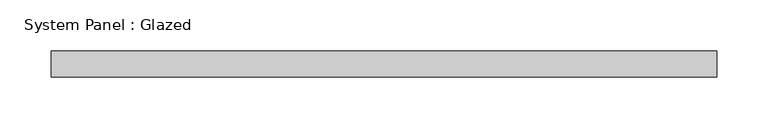
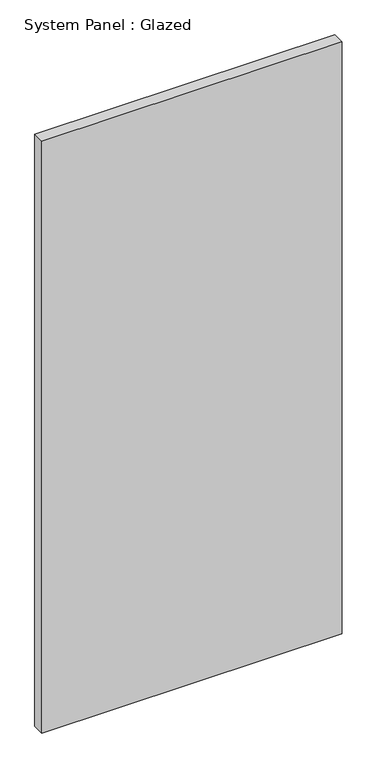
"""IFC4 building model written with IfcOpenShell, lengths in millimetres: plate geometry, System Panel : Glazed."""

from ifc_helpers import new_model, si_unit, origin, origin_with_axes, place, context, project, spatial, polyline, outline, extrude, source, transform, mapped, element, save


def system_panel_glazed_a5c0bc7c(model_context):
    return source(origin(), model_context, "Body", "SweptSolid", [
        extrude(outline(polyline([(323.85, 19.05), (-323.85, 19.05), (-323.85, 44.45), (323.85, 44.45), (323.85, 19.05)])), origin_with_axes(), (0.0, 0.0, 1.0), 1348.8013618),
    ])


if __name__ == "__main__":
    model = new_model("IFC4")
    model_context = context("Model", 3, world=origin())
    ifc_project = project(units=[si_unit("LENGTHUNIT", "METRE", prefix="MILLI")], contexts=[model_context])
    site = spatial("IfcSite", under=ifc_project)
    building = spatial("IfcBuilding", under=site)
    placement = place(None, origin())
    system_panel_glazed_shape = system_panel_glazed_a5c0bc7c(model_context)
    element("IfcPlate", 1, ObjectType="System Panel : Glazed", at=placement, inside=building, context=model_context, shape_type="MappedRepresentation", body=[
        mapped(system_panel_glazed_shape, transform((0.0, 0.0, 0.0), x_axis=(1.0, 0.0, 0.0), y_axis=(0.0, 1.0, 0.0), z_axis=(0.0, 0.0, 1.0))),
    ])
    save(model, "model.ifc")

# Revit data of these elements
# Type "System Panel : Glazed"
#   Construction Type Id = "GSP4R"
#   Analytic Construction = "1/8 in Pilkington single glazing"
#   Visual Light Transmittance = 0.9
#   Solar Heat Gain Coefficient = 0.86
#   Heat Transfer Coefficient (U) = 1.18115 BTU/(h·ft²·°F)
#   Define Thermal Properties by = 1
# Element 1 (IfcPlate, "System Panel : Glazed")
#   Materials on its faces: "Glass"
# Materials
#   "Glass": class "Glass", colour RGB 0 128 192, transparency 0.75, Description = "Soda Lime Glass", Cost = 0
